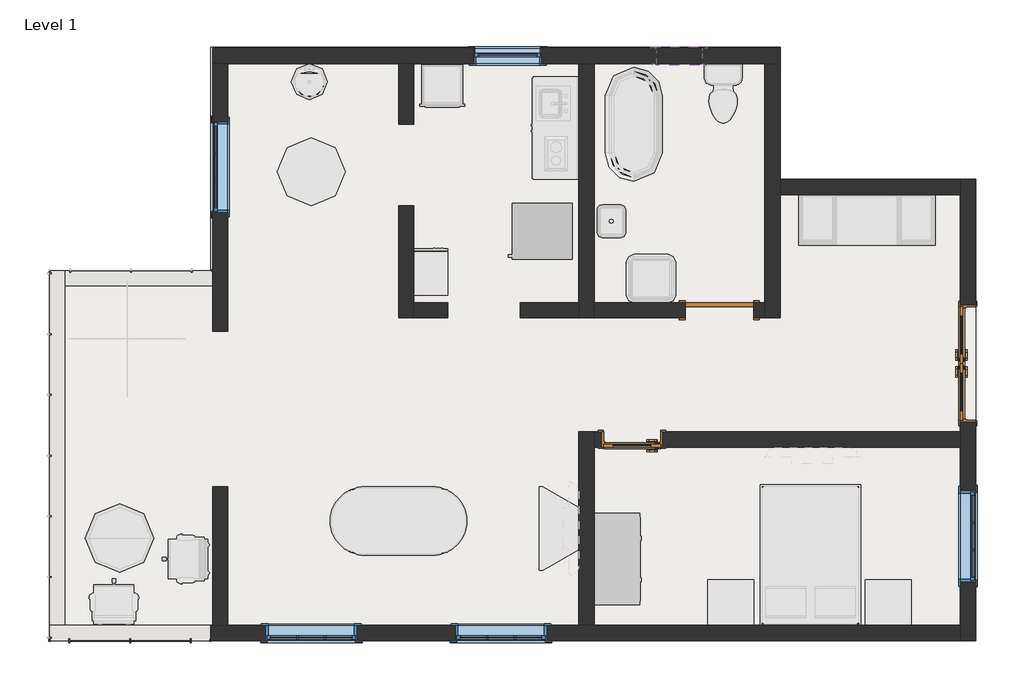
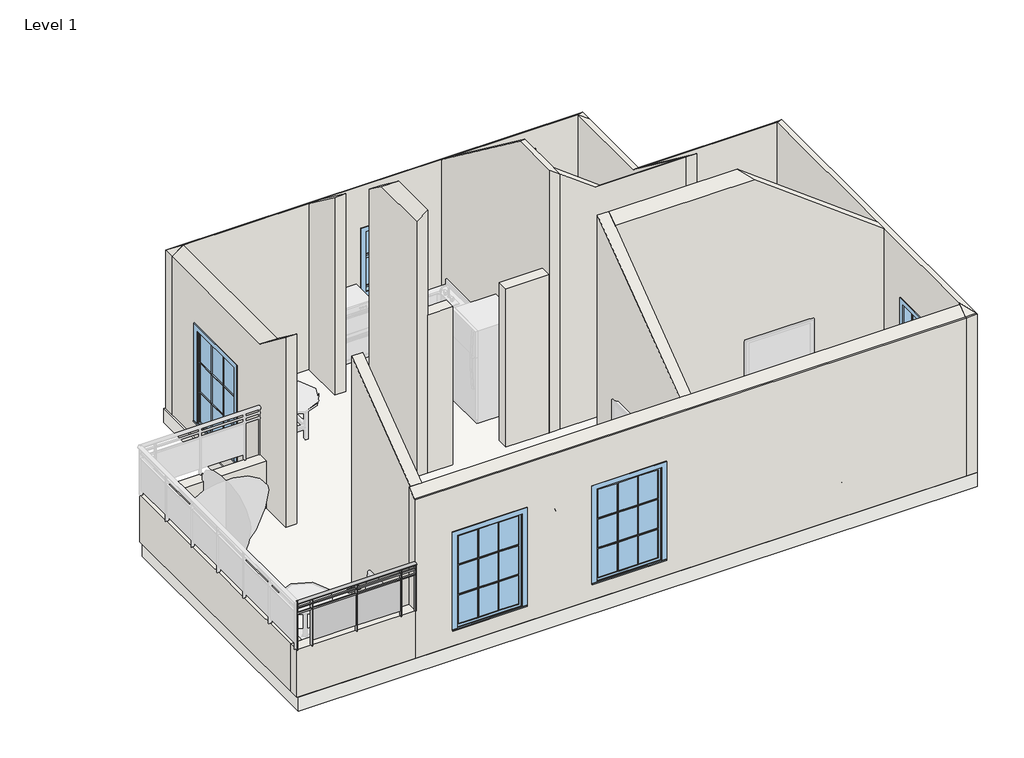
# One storey, part 1 of 2: 18 walls, 6 windows, 3 doors, 1 railing, 1 slab.
"""IFC4 building model written with IfcOpenShell, lengths in millimetres."""

from ifc_helpers import new_model, si_unit, point, frame, origin, origin_with_axes, place, context, project, spatial, polyline, ellipse_curve, trimmed, outline, extrude, faceted_brep, transform, mapped, element, save
from ifc_brep_helpers import plane_surface, extruded_surface, advanced_brep
from components import door_7e6851c9, door_b03bd389, door_54dd4da4, window_5a4e61ec, window_31198920, window_e41d21a6

model = new_model("IFC4")

# Units and contexts
model_context = context("Model", 3, world=origin())
ifc_project = project(units=[si_unit("LENGTHUNIT", "METRE", prefix="MILLI")], contexts=[model_context])

# Site, building, storey
site = spatial("IfcSite", under=ifc_project)
building = spatial("IfcBuilding", under=site)
storey = spatial("IfcBuildingStorey", under=building, Name="Level 1", Elevation=0.0)

# Doors
placement = place(None, origin())
door_shape = door_7e6851c9(model_context)
element("IfcDoor", 1, ObjectType="30\" x 80\"", at=placement, inside=storey, context=model_context, shape_type="MappedRepresentation", body=[
    mapped(door_shape, transform((-12235.0118725, 8691.4702409, 0.0), x_axis=(1.0, 0.0, 0.0), y_axis=(0.0, 1.0, 0.0), z_axis=(0.0, 0.0, 1.0))),
])
door_2_shape = door_b03bd389(model_context)
element("IfcDoor", 2, ObjectType="Door-Exterior-Double-Full Glass-Wood_Clad : 60\" x 80\"", at=placement, inside=storey, context=model_context, shape_type="MappedRepresentation", body=[
    mapped(door_2_shape, transform((-7742.3868725, 9710.6452409, 0.0), x_axis=(0.0, 1.0, 0.0), y_axis=(-1.0, 0.0, 0.0), z_axis=(0.0, 0.0, 1.0))),
])
door_3_shape = door_54dd4da4(model_context)
element("IfcDoor", 3, ObjectType="Single-Flush : 36\" x 84\"", at=placement, inside=storey, context=model_context, shape_type="MappedRepresentation", body=[
    mapped(door_3_shape, transform((-11066.6118725, 10421.8452409, 0.0), x_axis=(1.0, 0.0, 0.0), y_axis=(0.0, 1.0, 0.0), z_axis=(0.0, 0.0, 1.0))),
])

# Railing
element("IfcRailing", 4, ObjectType="Glass Panel - Bottom Fill", at=placement, inside=storey, context=model_context, shape_type="SolidModel", body=[
    advanced_brep(
    [(-17873.8118725, 5964.1452409, 1828.8), (-17873.8118725, 6040.3452409, 1828.8), (-20032.8118725, 5964.1452409, 1828.8), (-20032.8118725, 6040.3452409, 1828.8)],
    [
        (0, 1, ellipse_curve(frame((-17873.8118725, 6002.2452409, 1828.8), z_axis=(1.0, 0.0, 0.0), x_axis=(0.0, 1.0, 0.0)), 38.1, 28.575)),
        (1, 0, ellipse_curve(frame((-17873.8118725, 6002.2452409, 1828.8), z_axis=(1.0, 0.0, 0.0), x_axis=(0.0, 1.0, 0.0)), 38.1, 28.575)),
        (2, 3, ellipse_curve(frame((-20032.8118725, 6002.2452409, 1828.8), z_axis=(-1.0, 0.0, 0.0), x_axis=(0.0, 1.0, 0.0)), 38.1, 28.575)),
        (3, 2, ellipse_curve(frame((-20032.8118725, 6002.2452409, 1828.8), z_axis=(-1.0, 0.0, 0.0), x_axis=(0.0, 1.0, 0.0)), 38.1, 28.575)),
        (0, 2),
        (3, 1),
    ],
    [
        plane_surface(frame((-17873.8118725, 6002.2452409, 1828.8), z_axis=(1.0, 0.0, 0.0), x_axis=(0.0, -1.0, 0.0))),
        plane_surface(frame((-20032.8118725, 6002.2452409, 1828.8), z_axis=(-1.0, 0.0, 0.0), x_axis=(0.0, -1.0, 0.0))),
        extruded_surface(trimmed(ellipse_curve(frame((-20032.8118725, 6002.2452409, 1828.8), z_axis=(1.0, 0.0, 0.0), x_axis=(0.0, 1.0, 0.0)), 38.1, 28.575), [point((-20032.8118725, 5964.1452409, 1828.8))], [point((-20032.8118725, 6040.3452409, 1828.8))], True, "CARTESIAN"), (2159.0, 0.0, 0.0), 2159.0),
        extruded_surface(trimmed(ellipse_curve(frame((-20032.8118725, 6002.2452409, 1828.8), z_axis=(1.0, 0.0, 0.0), x_axis=(0.0, 1.0, 0.0)), 38.1, 28.575), [point((-20032.8118725, 6040.3452409, 1828.8))], [point((-20032.8118725, 5964.1452409, 1828.8))], True, "CARTESIAN"), (2159.0, 0.0, 0.0), 2159.0),
    ],
    [
        (0, [[1, 2]]),
        (1, [[3, 4]]),
        (2, [[-1, 5, -4, 6]]),
        (3, [[-2, -6, -3, -5]]),
    ],
),
    extrude(outline(polyline([(-17873.8118725, 6014.9452409), (-17873.8118725, 5989.5452409), (-20032.8118725, 5989.5452409), (-20032.8118725, 6014.9452409), (-17873.8118725, 6014.9452409)])), frame((0.0, 0.0, 1714.5), z_axis=(0.0, 0.0, 1.0), x_axis=(1.0, 0.0, 0.0)), (0.0, 0.0, 1.0), 25.4),
    extrude(outline(polyline([(-17873.8118725, 6014.9452409), (-17873.8118725, 5989.5452409), (-20032.8118725, 5989.5452409), (-20032.8118725, 6014.9452409), (-17873.8118725, 6014.9452409)])), frame((0.0, 0.0, 1612.9), z_axis=(0.0, 0.0, 1.0), x_axis=(1.0, 0.0, 0.0)), (0.0, 0.0, 1.0), 25.4),
    extrude(outline(polyline([(-19759.7618725, 6027.6452409), (-19759.7618725, 5976.8452409), (-19772.4618725, 5976.8452409), (-19772.4618725, 6027.6452409), (-19759.7618725, 6027.6452409)])), frame((0.0, 0.0, 914.4), z_axis=(0.0, 0.0, 1.0), x_axis=(1.0, 0.0, 0.0)), (0.0, 0.0, 1.0), 885.6788223),
    extrude(outline(polyline([(-18953.3118725, 5995.7100839), (-19766.1118725, 5995.7100839), (-19766.1118725, 6002.0600839), (-18953.3118725, 6002.0600839), (-18953.3118725, 5995.7100839)])), frame((0.0, 0.0, 1016.0), z_axis=(0.0, 0.0, 1.0), x_axis=(1.0, 0.0, 0.0)), (0.0, 0.0, 1.0), 596.9),
    extrude(outline(polyline([(-18946.9618725, 6027.6452409), (-18946.9618725, 5976.8452409), (-18959.6618725, 5976.8452409), (-18959.6618725, 6027.6452409), (-18946.9618725, 6027.6452409)])), frame((0.0, 0.0, 914.4), z_axis=(0.0, 0.0, 1.0), x_axis=(1.0, 0.0, 0.0)), (0.0, 0.0, 1.0), 885.6788223),
    extrude(outline(polyline([(-18140.5118725, 5995.7100839), (-18953.3118725, 5995.7100839), (-18953.3118725, 6002.0600839), (-18140.5118725, 6002.0600839), (-18140.5118725, 5995.7100839)])), frame((0.0, 0.0, 1016.0), z_axis=(0.0, 0.0, 1.0), x_axis=(1.0, 0.0, 0.0)), (0.0, 0.0, 1.0), 596.9),
    extrude(outline(polyline([(-18134.1618725, 6027.6452409), (-18134.1618725, 5976.8452409), (-18146.8618725, 5976.8452409), (-18146.8618725, 6027.6452409), (-18134.1618725, 6027.6452409)])), frame((0.0, 0.0, 914.4), z_axis=(0.0, 0.0, 1.0), x_axis=(1.0, 0.0, 0.0)), (0.0, 0.0, 1.0), 885.6788223),
    extrude(outline(polyline([(-20020.1118725, 6011.7702409), (-20020.1118725, 5992.7202409), (-20039.1618725, 5992.7202409), (-20039.1618725, 6011.7702409), (-20020.1118725, 6011.7702409)])), frame((0.0, 0.0, 914.4), z_axis=(0.0, 0.0, 1.0), x_axis=(1.0, 0.0, 0.0)), (0.0, 0.0, 1.0), 885.6788223),
    extrude(outline(polyline([(-17867.4618725, 6011.7702409), (-17867.4618725, 5992.7202409), (-17886.5118725, 5992.7202409), (-17886.5118725, 6011.7702409), (-17867.4618725, 6011.7702409)])), frame((0.0, 0.0, 914.4), z_axis=(0.0, 0.0, 1.0), x_axis=(1.0, 0.0, 0.0)), (0.0, 0.0, 1.0), 885.6788223),
])

# Slab
element("IfcSlab", 5, ObjectType="Wood Joist 10\" - Ceramic Tile", at=placement, inside=storey, context=model_context, shape_type="SweptSolid", body=[
    extrude(outline(polyline([(-20007.4118725, 10923.4952409), (-17873.8118725, 10923.4952409), (-17873.8118725, 13946.0952409), (-10253.8118725, 13946.0952409), (-10253.8118725, 12174.4452409), (-7637.6118725, 12174.4452409), (-7637.6118725, 10542.4952409), (-7637.6118725, 6002.2452409), (-20007.4118725, 6002.2452409), (-20007.4118725, 10923.4952409)])), frame((0.0, 0.0, -273.05), z_axis=(0.0, 0.0, 1.0), x_axis=(1.0, 0.0, 0.0)), (0.0, 0.0, 1.0), 273.05),
])

# Walls
element("IfcWall", 6, ObjectType="Generic - 8\"", at=placement, inside=storey, context=model_context, shape_type="Brep", body=[
    faceted_brep([(-7840.8118725, 6205.4452409, 0.0), (-12743.0118725, 6205.4452409, 0.0), (-12946.2118725, 6205.4452409, 0.0), (-17645.2118725, 6205.4452409, 0.0), (-17848.4118725, 6205.4452409, 0.0), (-17873.8118725, 6205.4452409, 0.0), (-17873.8118725, 6205.4452409, 914.4), (-17873.8118725, 6205.4452409, 3176.5875), (-17848.4118725, 6205.4452409, 3176.5875), (-17645.2118725, 6205.4452409, 3176.5875), (-12946.2118725, 6205.4452409, 3176.5875), (-12743.0118725, 6205.4452409, 3176.5875), (-7840.8118725, 6205.4452409, 3176.5875), (-17137.2118725, 6205.4452409, 2133.6), (-17137.2118725, 6205.4452409, 304.8), (-15918.0118725, 6205.4452409, 304.8), (-15918.0118725, 6205.4452409, 2133.6), (-14597.2118725, 6205.4452409, 2133.6), (-14597.2118725, 6205.4452409, 304.8), (-13378.0118725, 6205.4452409, 304.8), (-13378.0118725, 6205.4452409, 2133.6), (-7840.8118725, 6002.2452409, 0.0), (-7840.8118725, 6002.2452409, 3048.0), (-17873.8118725, 6002.2452409, 3048.0), (-17873.8118725, 6002.2452409, 914.4), (-17873.8118725, 6002.2452409, 0.0), (-17137.2118725, 6002.2452409, 2133.6), (-15918.0118725, 6002.2452409, 2133.6), (-15918.0118725, 6002.2452409, 304.8), (-17137.2118725, 6002.2452409, 304.8), (-14597.2118725, 6002.2452409, 2133.6), (-13378.0118725, 6002.2452409, 2133.6), (-13378.0118725, 6002.2452409, 304.8), (-14597.2118725, 6002.2452409, 304.8), (-17873.8118725, 6033.9952409, 3048.0), (-7840.8118725, 6033.9952409, 3048.0)], [[[0, 1, 2, 3, 4, 5, 6, 7, 8, 9, 10, 11, 12], [13, 14, 15, 16], [17, 18, 19, 20]], [[21, 22, 23, 24, 25], [26, 27, 28, 29], [30, 31, 32, 33]], [[5, 4, 3, 2, 1, 0, 21, 25]], [[7, 6, 5, 25, 24, 23, 34]], [[0, 12, 35, 22, 21]], [[34, 23, 22, 35]], [[12, 11, 10, 9, 8, 7, 34, 35]], [[14, 13, 26, 29]], [[15, 14, 29, 28]], [[16, 15, 28, 27]], [[13, 16, 27, 26]], [[18, 17, 30, 33]], [[19, 18, 33, 32]], [[20, 19, 32, 31]], [[17, 20, 31, 30]]]),
])
element("IfcWall", 7, ObjectType="Generic - 8\"", at=placement, inside=storey, context=model_context, shape_type="Brep", body=[
    faceted_brep([(-19829.6118725, 6205.4452409, 0.0), (-19829.6118725, 10752.0452409, 0.0), (-19829.6118725, 10955.2452409, 0.0), (-19829.6118725, 10955.2452409, 914.4), (-19829.6118725, 10752.0452409, 914.4), (-19829.6118725, 6205.4452409, 914.4), (-20032.8118725, 6205.4452409, 0.0), (-20032.8118725, 6205.4452409, 914.4), (-20032.8118725, 10955.2452409, 914.4), (-20032.8118725, 10955.2452409, 0.0)], [[[0, 1, 2, 3, 4, 5]], [[6, 7, 8, 9]], [[2, 1, 0, 6, 9]], [[5, 4, 3, 8, 7]], [[0, 5, 7, 6]], [[3, 2, 9, 8]]]),
])
element("IfcWall", 8, ObjectType="Generic - 8\"", at=placement, inside=storey, context=model_context, shape_type="SweptSolid", body=[
    extrude(outline(polyline([(12174.4452409, 3048.0), (12174.4452409, 0.0), (11971.2452409, 0.0), (11971.2452409, 3200.4), (12174.4452409, 3048.0)])), frame((-10253.8118725, 0.0, 0.0), z_axis=(1.0, 0.0, 0.0), x_axis=(0.0, 1.0, 0.0)), (0.0, 0.0, 1.0), 2413.0),
])
element("IfcWall", 9, ObjectType="Generic - 8\"", at=placement, inside=storey, context=model_context, shape_type="Brep", body=[
    faceted_brep([(-10253.8118725, 10320.2452409, 0.0), (-10253.8118725, 11971.2452409, 0.0), (-10253.8118725, 12174.4452409, 0.0), (-10253.8118725, 13723.8452409, 0.0), (-10253.8118725, 13723.8452409, 3048.0), (-10253.8118725, 12174.4452409, 3048.0), (-10253.8118725, 11971.2452409, 3200.4), (-10253.8118725, 10320.2452409, 4438.65), (-10457.0118725, 10320.2452409, 0.0), (-10457.0118725, 10320.2452409, 4438.65), (-10457.0118725, 10523.4452409, 4286.25), (-10457.0118725, 11971.2452409, 3200.4), (-10457.0118725, 13723.8452409, 3200.4), (-10457.0118725, 13723.8452409, 0.0), (-10457.0118725, 10523.4452409, 0.0)], [[[0, 1, 2, 3, 4, 5, 6, 7]], [[8, 9, 10, 11, 12, 13, 14]], [[3, 2, 1, 0, 8, 14, 13]], [[4, 3, 13, 12]], [[0, 7, 9, 8]], [[7, 6, 5, 11, 10, 9]], [[5, 4, 12, 11]]]),
])
element("IfcWall", 10, ObjectType="Generic - 8\"", at=placement, inside=storey, context=model_context, shape_type="Brep", body=[
    faceted_brep([(-12946.2118725, 13723.8452409, 0.0), (-12946.2118725, 10523.4452409, 0.0), (-12946.2118725, 10320.2452409, 0.0), (-12946.2118725, 10320.2452409, 3048.0), (-12946.2118725, 10320.2452409, 5067.3), (-12946.2118725, 11234.6452409, 5067.3), (-12946.2118725, 13723.8452409, 3200.4), (-12743.0118725, 13723.8452409, 0.0), (-12743.0118725, 13723.8452409, 3200.4), (-12743.0118725, 11437.8452409, 4914.9), (-12743.0118725, 10523.4452409, 4914.9), (-12743.0118725, 10320.2452409, 4914.9), (-12743.0118725, 10320.2452409, 0.0), (-12743.0118725, 10523.4452409, 0.0)], [[[0, 1, 2, 3, 4, 5, 6]], [[7, 8, 9, 10, 11, 12, 13]], [[2, 1, 0, 7, 13, 12]], [[0, 6, 8, 7]], [[6, 5, 9, 8]], [[5, 4, 11, 10, 9]], [[4, 3, 2, 12, 11]]]),
])
element("IfcWall", 11, ObjectType="Generic - 8\"", at=placement, inside=storey, context=model_context, shape_type="Brep", body=[
    faceted_brep([(-17848.4118725, 13723.8452409, 0.0), (-17848.4118725, 10955.2452409, 0.0), (-17848.4118725, 10752.0452409, 0.0), (-17848.4118725, 10142.4452409, 0.0), (-17848.4118725, 10142.4452409, 3657.6), (-17848.4118725, 10955.2452409, 3048.0), (-17848.4118725, 13723.8452409, 3048.0), (-17848.4118725, 12949.1452409, 2133.6), (-17848.4118725, 11729.9452409, 2133.6), (-17848.4118725, 11729.9452409, 304.8), (-17848.4118725, 12949.1452409, 304.8), (-17645.2118725, 13723.8452409, 0.0), (-17645.2118725, 13723.8452409, 3200.4), (-17645.2118725, 10752.0452409, 3200.4), (-17645.2118725, 10142.4452409, 3657.6), (-17645.2118725, 10142.4452409, 0.0), (-17645.2118725, 12949.1452409, 2133.6), (-17645.2118725, 12949.1452409, 304.8), (-17645.2118725, 11729.9452409, 304.8), (-17645.2118725, 11729.9452409, 2133.6)], [[[0, 1, 2, 3, 4, 5, 6], [7, 8, 9, 10]], [[11, 12, 13, 14, 15], [16, 17, 18, 19]], [[3, 2, 1, 0, 11, 15]], [[4, 3, 15, 14]], [[0, 6, 12, 11]], [[6, 5, 13, 12]], [[5, 4, 14, 13]], [[17, 16, 7, 10]], [[18, 17, 10, 9]], [[19, 18, 9, 8]], [[16, 19, 8, 7]]]),
])
element("IfcWall", 12, ObjectType="Generic - 8\"", at=placement, inside=storey, context=model_context, shape_type="SweptSolid", body=[
    extrude(outline(polyline([(-19829.6118725, 10955.2452409), (-17848.4118725, 10955.2452409), (-17848.4118725, 10752.0452409), (-19829.6118725, 10752.0452409), (-19829.6118725, 10955.2452409)])), origin_with_axes(), (0.0, 0.0, 1.0), 914.4),
])
element("IfcWall", 13, ObjectType="Generic - 8\"", at=placement, inside=storey, context=model_context, shape_type="Brep", body=[
    faceted_brep([(-17848.4118725, 13723.8452409, 0.0), (-17645.2118725, 13723.8452409, 0.0), (-15359.2118725, 13723.8452409, 0.0), (-15156.0118725, 13723.8452409, 0.0), (-12946.2118725, 13723.8452409, 0.0), (-12743.0118725, 13723.8452409, 0.0), (-10457.0118725, 13723.8452409, 0.0), (-10253.8118725, 13723.8452409, 0.0), (-10253.8118725, 13723.8452409, 3048.0), (-10457.0118725, 13723.8452409, 3200.4), (-12743.0118725, 13723.8452409, 3200.4), (-12946.2118725, 13723.8452409, 3200.4), (-15156.0118725, 13723.8452409, 3200.4), (-15359.2118725, 13723.8452409, 3200.4), (-17645.2118725, 13723.8452409, 3200.4), (-17848.4118725, 13723.8452409, 3048.0), (-13441.5118725, 13723.8452409, 2336.8), (-13441.5118725, 13723.8452409, 1117.6), (-14355.9118725, 13723.8452409, 1117.6), (-14355.9118725, 13723.8452409, 2336.8), (-11295.2118725, 13723.8452409, 2768.6), (-11295.2118725, 13723.8452409, 2159.0), (-11904.8118725, 13723.8452409, 2159.0), (-11904.8118725, 13723.8452409, 2768.6), (-17848.4118725, 13927.0452409, 0.0), (-17848.4118725, 13927.0452409, 3048.0), (-10253.8118725, 13927.0452409, 3048.0), (-10253.8118725, 13927.0452409, 0.0), (-13441.5118725, 13927.0452409, 2336.8), (-14355.9118725, 13927.0452409, 2336.8), (-14355.9118725, 13927.0452409, 1117.6), (-13441.5118725, 13927.0452409, 1117.6), (-11295.2118725, 13927.0452409, 2768.6), (-11904.8118725, 13927.0452409, 2768.6), (-11904.8118725, 13927.0452409, 2159.0), (-11295.2118725, 13927.0452409, 2159.0)], [[[0, 1, 2, 3, 4, 5, 6, 7, 8, 9, 10, 11, 12, 13, 14, 15], [16, 17, 18, 19], [20, 21, 22, 23]], [[24, 25, 26, 27], [28, 29, 30, 31], [32, 33, 34, 35]], [[7, 6, 5, 4, 3, 2, 1, 0, 24, 27]], [[0, 15, 25, 24]], [[8, 7, 27, 26]], [[15, 14, 25]], [[14, 13, 12, 11, 10, 9, 26, 25]], [[9, 8, 26]], [[17, 16, 28, 31]], [[18, 17, 31, 30]], [[19, 18, 30, 29]], [[16, 19, 29, 28]], [[21, 20, 32, 35]], [[22, 21, 35, 34]], [[23, 22, 34, 33]], [[20, 23, 33, 32]]]),
])
element("IfcWall", 14, ObjectType="Generic - 8\"", at=placement, inside=storey, context=model_context, shape_type="Brep", body=[
    faceted_brep([(-7840.8118725, 6002.2452409, 0.0), (-7840.8118725, 6002.2452409, 3048.0), (-7840.8118725, 6033.9952409, 3048.0), (-7840.8118725, 6205.4452409, 3176.5875), (-7840.8118725, 6237.1952409, 3200.4), (-7840.8118725, 8593.0452409, 3200.4), (-7840.8118725, 8796.2452409, 3200.4), (-7840.8118725, 11971.2452409, 3200.4), (-7840.8118725, 12174.4452409, 3048.0), (-7840.8118725, 12174.4452409, 0.0), (-7840.8118725, 11971.2452409, 0.0), (-7840.8118725, 10498.0452409, 0.0), (-7840.8118725, 10498.0452409, 2057.4), (-7840.8118725, 8923.2452409, 2057.4), (-7840.8118725, 8923.2452409, 0.0), (-7840.8118725, 8796.2452409, 0.0), (-7840.8118725, 8593.0452409, 0.0), (-7840.8118725, 6205.4452409, 0.0), (-7840.8118725, 6789.6452409, 2133.6), (-7840.8118725, 6789.6452409, 304.8), (-7840.8118725, 8008.8452409, 304.8), (-7840.8118725, 8008.8452409, 2133.6), (-7637.6118725, 6002.2452409, 3048.0), (-7637.6118725, 6002.2452409, 0.0), (-7637.6118725, 8923.2452409, 0.0), (-7637.6118725, 8923.2452409, 2057.4), (-7637.6118725, 10498.0452409, 2057.4), (-7637.6118725, 10498.0452409, 0.0), (-7637.6118725, 12174.4452409, 0.0), (-7637.6118725, 12174.4452409, 3048.0), (-7637.6118725, 6033.9952409, 3048.0), (-7637.6118725, 6789.6452409, 2133.6), (-7637.6118725, 8008.8452409, 2133.6), (-7637.6118725, 8008.8452409, 304.8), (-7637.6118725, 6789.6452409, 304.8)], [[[0, 1, 2, 3, 4, 5, 6, 7, 8, 9, 10, 11, 12, 13, 14, 15, 16, 17], [18, 19, 20, 21]], [[22, 23, 24, 25, 26, 27, 28, 29, 30], [31, 32, 33, 34]], [[23, 0, 17, 16, 15, 14, 24]], [[9, 28, 27, 11, 10]], [[1, 0, 23, 22]], [[9, 8, 29, 28]], [[26, 12, 11, 27]], [[12, 26, 25, 13]], [[13, 25, 24, 14]], [[1, 22, 30, 2]], [[29, 8, 7]], [[30, 29, 7, 6, 5, 4]], [[4, 3, 2, 30]], [[19, 18, 31, 34]], [[20, 19, 34, 33]], [[21, 20, 33, 32]], [[18, 21, 32, 31]]]),
])
element("IfcWall", 15, ObjectType="Generic - 8\"", at=placement, inside=storey, context=model_context, shape_type="Brep", body=[
    faceted_brep([(-12743.0118725, 8593.0452409, 4967.2875), (-12743.0118725, 8593.0452409, 0.0), (-12641.4118725, 8593.0452409, 0.0), (-12641.4118725, 8593.0452409, 2057.4), (-11828.6118725, 8593.0452409, 2057.4), (-11828.6118725, 8593.0452409, 0.0), (-7840.8118725, 8593.0452409, 0.0), (-7840.8118725, 8593.0452409, 3200.4), (-10196.6618725, 8593.0452409, 4967.2875), (-12743.0118725, 8796.2452409, 0.0), (-12743.0118725, 8796.2452409, 5119.6875), (-10399.8618725, 8796.2452409, 5119.6875), (-7840.8118725, 8796.2452409, 3200.4), (-7840.8118725, 8796.2452409, 0.0), (-11828.6118725, 8796.2452409, 0.0), (-11828.6118725, 8796.2452409, 2057.4), (-12641.4118725, 8796.2452409, 2057.4), (-12641.4118725, 8796.2452409, 0.0)], [[[0, 1, 2, 3, 4, 5, 6, 7, 8]], [[9, 10, 11, 12, 13, 14, 15, 16, 17]], [[1, 9, 17, 2]], [[13, 6, 5, 14]], [[1, 0, 10, 9]], [[7, 6, 13, 12]], [[4, 15, 14, 5]], [[15, 4, 3, 16]], [[16, 3, 2, 17]], [[10, 0, 8, 11]], [[7, 12, 11, 8]]]),
])
element("IfcWall", 16, ObjectType="Generic - 8\"", at=placement, inside=storey, context=model_context, shape_type="Brep", body=[
    faceted_brep([(-10609.4118725, 10320.2452409, 2133.6), (-10609.4118725, 10320.2452409, 0.0), (-10457.0118725, 10320.2452409, 0.0), (-10457.0118725, 10320.2452409, 4438.65), (-12108.0118725, 10320.2452409, 4438.65), (-12743.0118725, 10320.2452409, 4914.9), (-12743.0118725, 10320.2452409, 0.0), (-11523.8118725, 10320.2452409, 0.0), (-11523.8118725, 10320.2452409, 2133.6), (-10457.0118725, 10523.4452409, 0.0), (-10609.4118725, 10523.4452409, 0.0), (-10609.4118725, 10523.4452409, 2133.6), (-11523.8118725, 10523.4452409, 2133.6), (-11523.8118725, 10523.4452409, 0.0), (-12743.0118725, 10523.4452409, 0.0), (-12743.0118725, 10523.4452409, 4914.9), (-11904.8118725, 10523.4452409, 4286.25), (-10457.0118725, 10523.4452409, 4286.25)], [[[0, 1, 2, 3, 4, 5, 6, 7, 8]], [[9, 10, 11, 12, 13, 14, 15, 16, 17]], [[7, 6, 14, 13]], [[2, 1, 10, 9]], [[3, 2, 9, 17]], [[6, 5, 15, 14]], [[11, 10, 1, 0]], [[12, 11, 0, 8]], [[13, 12, 8, 7]], [[5, 4, 16, 15]], [[4, 3, 17, 16]]]),
])
element("IfcWall", 17, ObjectType="Generic - 8\"", at=placement, inside=storey, context=model_context, shape_type="SweptSolid", body=[
    extrude(outline(polyline([(13723.8452409, 0.0), (12911.0452409, 0.0), (12911.0452409, 3810.0), (13723.8452409, 3200.4), (13723.8452409, 0.0)])), frame((-15359.2118725, 0.0, 0.0), z_axis=(1.0, 0.0, 0.0), x_axis=(0.0, 1.0, 0.0)), (0.0, 0.0, 1.0), 203.2),
])
element("IfcWall", 18, ObjectType="Generic - 8\"", at=placement, inside=storey, context=model_context, shape_type="Brep", body=[
    faceted_brep([(-15359.2118725, 11818.8452409, 0.0), (-15359.2118725, 10320.2452409, 0.0), (-15359.2118725, 10320.2452409, 4914.9), (-15359.2118725, 11437.8452409, 4914.9), (-15359.2118725, 11818.8452409, 4629.15), (-15156.0118725, 11818.8452409, 0.0), (-15156.0118725, 11818.8452409, 4629.15), (-15156.0118725, 11234.6452409, 5067.3), (-15156.0118725, 10320.2452409, 5067.3), (-15156.0118725, 10320.2452409, 3048.0), (-15156.0118725, 10320.2452409, 0.0), (-15156.0118725, 10523.4452409, 0.0)], [[[0, 1, 2, 3, 4]], [[5, 6, 7, 8, 9, 10, 11]], [[1, 0, 5, 11, 10]], [[0, 4, 6, 5]], [[2, 1, 10, 9, 8]], [[4, 3, 7, 6]], [[3, 2, 8, 7]]]),
])
element("IfcWall", 19, ObjectType="Generic - 8\"", at=placement, inside=storey, context=model_context, shape_type="Brep", body=[
    faceted_brep([(-17873.8118725, 6205.4452409, 0.0), (-19829.6118725, 6205.4452409, 0.0), (-20032.8118725, 6205.4452409, 0.0), (-20032.8118725, 6205.4452409, 914.4), (-19829.6118725, 6205.4452409, 914.4), (-17873.8118725, 6205.4452409, 914.4), (-17873.8118725, 6002.2452409, 0.0), (-17873.8118725, 6002.2452409, 914.4), (-20032.8118725, 6002.2452409, 914.4), (-20032.8118725, 6002.2452409, 0.0)], [[[0, 1, 2, 3, 4, 5]], [[6, 7, 8, 9]], [[2, 1, 0, 6, 9]], [[5, 4, 3, 8, 7]], [[0, 5, 7, 6]], [[3, 2, 9, 8]]]),
])
element("IfcWall", 20, ObjectType="Generic - 8\"", at=placement, inside=storey, context=model_context, shape_type="SweptSolid", body=[
    extrude(outline(polyline([(8059.6452409, 0.0), (6205.4452409, 0.0), (6205.4452409, 3176.5875), (8059.6452409, 4567.2375), (8059.6452409, 0.0)])), frame((-17848.4118725, 0.0, 0.0), z_axis=(1.0, 0.0, 0.0), x_axis=(0.0, 1.0, 0.0)), (0.0, 0.0, 1.0), 203.2),
])
element("IfcWall", 21, ObjectType="Generic - 8\"", at=placement, inside=storey, context=model_context, shape_type="Brep", body=[
    faceted_brep([(-12946.2118725, 8796.2452409, 0.0), (-12946.2118725, 6205.4452409, 0.0), (-12946.2118725, 6205.4452409, 3176.5875), (-12946.2118725, 8796.2452409, 5119.6875), (-12743.0118725, 8796.2452409, 0.0), (-12743.0118725, 8796.2452409, 5119.6875), (-12743.0118725, 8593.0452409, 4967.2875), (-12743.0118725, 6205.4452409, 3176.5875), (-12743.0118725, 6205.4452409, 0.0), (-12743.0118725, 8593.0452409, 0.0)], [[[0, 1, 2, 3]], [[4, 5, 6, 7, 8, 9]], [[1, 0, 4, 9, 8]], [[0, 3, 5, 4]], [[2, 1, 8, 7]], [[3, 2, 7, 6, 5]]]),
])
element("IfcWall", 22, ObjectType="Generic - 8\"", at=placement, inside=storey, context=model_context, shape_type="SweptSolid", body=[
    extrude(outline(polyline([(-13733.6118725, 10523.4452409), (-12946.2118725, 10523.4452409), (-12946.2118725, 10320.2452409), (-13733.6118725, 10320.2452409), (-13733.6118725, 10523.4452409)])), origin_with_axes(), (0.0, 0.0, 1.0), 3048.0),
])
element("IfcWall", 23, ObjectType="Generic - 8\"", at=placement, inside=storey, context=model_context, shape_type="SweptSolid", body=[
    extrude(outline(polyline([(-15156.0118725, 10523.4452409), (-14698.8118725, 10523.4452409), (-14698.8118725, 10320.2452409), (-15156.0118725, 10320.2452409), (-15156.0118725, 10523.4452409)])), origin_with_axes(), (0.0, 0.0, 1.0), 3048.0),
])

# Windows
window_shape = window_5a4e61ec(model_context)
element("IfcWindow", 24, ObjectType="Casement 3x3 with Trim : 48\" x 72\"", at=placement, inside=storey, context=model_context, shape_type="MappedRepresentation", body=[
    mapped(window_shape, transform((-16527.6118725, 6103.8452409, 0.0), x_axis=(-1.0, 0.0, 0.0), y_axis=(0.0, -1.0, 0.0), z_axis=(0.0, 0.0, 1.0))),
])
element("IfcWindow", 25, ObjectType="Casement 3x3 with Trim : 48\" x 72\"", at=placement, inside=storey, context=model_context, shape_type="MappedRepresentation", body=[
    mapped(window_shape, transform((-13987.6118725, 6103.8452409, 0.0), x_axis=(-1.0, 0.0, 0.0), y_axis=(0.0, -1.0, 0.0), z_axis=(0.0, 0.0, 1.0))),
])
element("IfcWindow", 26, ObjectType="Casement 3x3 with Trim : 48\" x 72\"", at=placement, inside=storey, context=model_context, shape_type="MappedRepresentation", body=[
    mapped(window_shape, transform((-7739.2118725, 7399.2452409, 0.0), x_axis=(0.0, -1.0, 0.0), y_axis=(1.0, 0.0, 0.0), z_axis=(0.0, 0.0, 1.0))),
])
element("IfcWindow", 27, ObjectType="Casement 3x3 with Trim : 48\" x 72\"", at=placement, inside=storey, context=model_context, shape_type="MappedRepresentation", body=[
    mapped(window_shape, transform((-17746.8118725, 12339.5452409, 0.0), x_axis=(0.0, 1.0, 0.0), y_axis=(-1.0, 0.0, 0.0), z_axis=(0.0, 0.0, 1.0))),
])
window_2_shape = window_31198920(model_context)
element("IfcWindow", 28, ObjectType="Double Hung with Trim : 36\" x 48\"", at=placement, inside=storey, context=model_context, shape_type="MappedRepresentation", body=[
    mapped(window_2_shape, transform((-13898.7118725, 13825.4452409, 203.2), x_axis=(1.0, 0.0, 0.0), y_axis=(0.0, 1.0, 0.0), z_axis=(0.0, 0.0, 1.0))),
])
window_3_shape = window_e41d21a6(model_context)
element("IfcWindow", 29, ObjectType="Transom with Trim : 24\" x 24\"", at=placement, inside=storey, context=model_context, shape_type="MappedRepresentation", body=[
    mapped(window_3_shape, transform((-11561.9118725, 13825.4452409, 0.0), x_axis=(1.0, 0.0, 0.0), y_axis=(0.0, 1.0, 0.0), z_axis=(0.0, 0.0, 1.0))),
])

save(model, "model.ifc")

# Revit data of these elements
# Type "30\" x 80\""
#   Type Mark = "9"
#   Assembly Code = "B2030100"
#   Analytic Construction = "French door, wood frame with single glass"
#   Top Rail = 0' - 4 3/4"
#   Threshold Offset [instance default] = 0' - 0 1/2"
#   Thickness = 0' - 1 3/8"
#   Thermal Resistance (R) = 1.0696 (h·ft²·°F)/BTU
#   Swing Angle [instance default] = 90.00°
#   Stiles = 0' - 4 3/4"
#   Rough Width = 2' - 8"
#   Rough Height = 6' - 9"
#   Lock Rail = 0' - 7 1/8"
#   Height = 6' - 8"
#   Width = 2' - 6"
#   Heat Transfer Coefficient (U) = 0.9350 BTU/(h·ft²·°F)
#   Door Offset [instance default] = 0' - 0"
#   Bottom Rail = 0' - 9 1/2"
#   Threshold [instance default] = yes
#   Function = 1
#   Exterior Trim [instance default] = yes
#   Trim Material = Cherry
#   Threshold Material = Cherry
#   Panel Material = Cherry
#   Glazing = Glass
#   Frame Material = Cherry
#   Door Handle Material = Aluminum
#   Visual Light Transmittance = 0
#   Solar Heat Gain Coefficient = 0
#   Wall Closure = (empty or 0)
#   Construction Type = (empty or 0)
# Type "Door-Exterior-Double-Full Glass-Wood_Clad : 60\" x 80\""
#   Type Mark = "8"
#   Assembly Code = "B2030100"
#   Analytic Construction = "French door, wood frame with double glass"
#   Top Rail = 0' - 4 11/16"
#   Threshold Offset [instance default] = 0' - 0 1/2"
#   Thickness = 0' - 1 3/8"
#   Thermal Resistance (R) = 1.9158 (h·ft²·°F)/BTU
#   Swing Angle [instance default] = 90.00°
#   Stiles = 0' - 4 3/4"
#   Rough Width = 5' - 2"
#   Rough Height = 6' - 9"
#   Panel Width = 2' - 6"
#   Door Offset [instance default] = 0' - 0"
#   Height = 6' - 8"
#   Width = 5' - 0"
#   Heat Transfer Coefficient (U) = 0.5220 BTU/(h·ft²·°F)
#   Bottom Rail = 0' - 9 1/8"
#   Exterior Trim [instance default] = yes
#   Threshold [instance default] = yes
#   Show Grill [instance default] = yes
#   Function = 1
#   Trim Material = Cherry
#   Threshold Material = Cherry
#   Panel Material = Cherry
#   Glazing = Glass
#   Frame Material = Cherry
#   Door Handle Material = Aluminum
#   Visual Light Transmittance = 0
#   Solar Heat Gain Coefficient = 0
#   Wall Closure = (empty or 0)
#   Construction Type = (empty or 0)
# Type "Single-Flush : 36\" x 84\""
#   Type Mark = "1"
#   Construction Type Id = "MDOOR"
#   Assembly Code = "C1020"
#   Analytic Construction = "Metal"
#   Thickness = 0' - 2"
#   Heat Transfer Coefficient (U) = 0.651978 BTU/(h·ft²·°F)
#   Height = 7' - 0"
#   Trim Projection Ext = 0' - 1"
#   Trim Projection Int = 0' - 1"
#   Trim Width = 0' - 3"
#   Width = 3' - 0"
#   Define Thermal Properties by = 1
#   Door Material = Door - Panel
#   Frame Material = Door - Frame
#   Visual Light Transmittance = 0
#   Solar Heat Gain Coefficient = 0
#   Function = (empty or 0)
#   Wall Closure = (empty or 0)
# Type "Glass Panel - Bottom Fill"
#   Assembly Code = "C2010400"
#   built-in parameter 1008612 = 0.0416667 (stored number, unit not read)
#   built-in parameter 1008611 = 0.0416667 (stored number, unit not read)
#   built-in parameter 1008609 = 0.333333 (stored number, unit not read)
#   built-in parameter 1008604 = 0.166667 (stored number, unit not read)
#   built-in parameter 1008603 = 0.166667 (stored number, unit not read)
#   Railing Height = 3' - 0"
#   built-in parameter 1008630 = 2
#   built-in parameter 1008610 = 2
#   built-in parameter 1008618 = Baluster - Square : 3/4"
# Type "Wood Joist 10\" - Ceramic Tile"
#   Assembly Code = "B1010"
#   Function = 0
#   Layers, outside or top first: 0' - 0 1/4" "Tile, Mosaic, Gray" (function 5); 0' - 0 1/2" "Concrete, Cast-in-Place gray" (function 4); 0' - 0 3/4" "Plywood, Sheathing" (function 1); 0' - 9 1/4" "Structure, Wood Joist/Rafter Layer" (function 1)
# Type "Generic - 8\""
#   Assembly Code = "B2010"
#   Layers, outside or top first: 0' - 8" "Brick, Common" (function 1)
# Type "Casement 3x3 with Trim : 48\" x 72\""
#   Type Mark = "12"
#   Construction Type Id = "GSP4R"
#   Assembly Code = "B2020100"
#   Analytic Construction = "1/8 in Pilkington single glazing"
#   Visual Light Transmittance = 0.9
#   Solar Heat Gain Coefficient = 0.78
#   Heat Transfer Coefficient (U) = 0.6496 BTU/(h·ft²·°F)
#   Height = 6' - 0"
#   Default Sill Height = 1' - 0"
#   Trim Projection - Ext. = 0' - 0 1/2"
#   Trim Projection - Int. = 0' - 0 3/4"
#   Trim Width - Exterior = 0' - 3 1/2"
#   Trim Width - Interior = 0' - 3 1/2"
#   Width = 4' - 0"
#   Window Inset = 0' - 0 3/4"
#   Define Thermal Properties by = 1
#   Glass Pane Material = Glass
#   Sash Material = Sash
#   Trim Exterior Material = Trim
#   Trim Interior Material = Trim
#   Wall Closure = (empty or 0)
# Type "Double Hung with Trim : 36\" x 48\""
#   Type Mark = "13"
#   Construction Type Id = "GSP4R"
#   Assembly Code = "B2020100"
#   Analytic Construction = "1/8 in Pilkington single glazing"
#   Visual Light Transmittance = 0.9
#   Solar Heat Gain Coefficient = 0.78
#   Heat Transfer Coefficient (U) = 0.6496 BTU/(h·ft²·°F)
#   Height = 4' - 0"
#   Default Sill Height = 3' - 0"
#   Trim Projection - Ext. = 0' - 0 1/2"
#   Trim Projection - Int. = 0' - 0 3/4"
#   Trim Width - Exterior = 0' - 3 1/2"
#   Trim Width - Interior = 0' - 3 1/2"
#   Width = 3' - 0"
#   Window Inset = 0' - 0 3/4"
#   Define Thermal Properties by = 1
#   Glass Pane Material = Glass
#   Sash Material = Sash
#   Trim Exterior Material = Trim
#   Trim Interior Material = Trim
#   Wall Closure = (empty or 0)
# Type "Transom with Trim : 24\" x 24\""
#   Type Mark = "22"
#   Construction Type Id = "GSP4R"
#   Assembly Code = "B2020100"
#   Analytic Construction = "1/8 in Pilkington single glazing"
#   Visual Light Transmittance = 0.9
#   Solar Heat Gain Coefficient = 0.78
#   Heat Transfer Coefficient (U) = 0.6496 BTU/(h·ft²·°F)
#   Height = 2' - 0"
#   Default Sill Height = 7' - 1"
#   Trim Projection - Ext. = 0' - 0 1/2"
#   Trim Projection - Int. = 0' - 0 3/4"
#   Trim Width - Exterior = 0' - 3 1/2"
#   Trim Width - Interior = 0' - 3 1/2"
#   Width = 2' - 0"
#   Window Inset = 0' - 0 3/4"
#   Define Thermal Properties by = 1
#   Glass Pane Material = Glass
#   Sash Material = Sash
#   Trim Exterior Material = Trim
#   Trim Interior Material = Trim
#   Wall Closure = (empty or 0)
# Element 1 (IfcDoor, "30\" x 80\"")
#   Threshold Offset = 0' - 0 1/2"
#   Swing Angle = 90.00°
#   Door Offset = 0' - 0"
#   Threshold = yes
#   Exterior Trim = yes
#   Phase Created = New Construction
#   Materials on its faces: "Cherry", "Aluminum", "Glass"
# Element 2 (IfcDoor, "Door-Exterior-Double-Full Glass-Wood_Clad : 60\" x 80\"")
#   Threshold Offset = 0' - 0 1/2"
#   Swing Angle = 90.00°
#   Door Offset = 0' - 0"
#   Threshold = yes
#   Show Grill = yes
#   Exterior Trim = yes
#   Phase Created = New Construction
#   Materials on its faces: "Cherry", "Aluminum", "Glass"
# Element 3 (IfcDoor, "Single-Flush : 36\" x 84\"")
#   Phase Created = New Construction
#   Materials on its faces: "Door - Frame", "Door - Panel"
# Element 4 (IfcRailing, "Glass Panel - Bottom Fill")
#   built-in parameter 1008621 = 3 (stored number, unit not read)
#   Phase Created = New Construction
#   Materials on its faces: "Glass"
# Element 5 (IfcSlab, "Wood Joist 10\" - Ceramic Tile")
#   built-in parameter 1001955 = 1.5708 (stored number, unit not read)
#   Height Offset From Level = 0' - 0"
#   Phase Created = New Construction
#   Materials on its faces: "Structure, Wood Joist/Rafter Layer", "Tile, Mosaic, Gray"
# Elements 6, 8, 9, 10, 11, 13, 14, 15, 16, 17, 18, 20, 21, 22, 23 (IfcWall, "Generic - 8\"")
#   Top Offset = 0' - 0"
#   Base Offset = 0' - 0"
#   Unconnected Height = 10' - 0"
#   wall height = 10' - 0"
#   Phase Created = New Construction
#   Base Constraint = Level 1
#   Materials on its faces: "Brick, Common"
# Elements 7, 12, 19 (IfcWall, "Generic - 8\"")
#   Top Offset = 0' - 0"
#   Base Offset = 0' - 0"
#   Unconnected Height = 3' - 0"
#   wall height = 3' - 0"
#   Phase Created = New Construction
#   Base Constraint = Level 1
#   Materials on its faces: "Brick, Common"
# Element 24 (IfcWindow, "Casement 3x3 with Trim : 48\" x 72\"")
#   Mark = "1"
#   Phase Created = New Construction
#   Materials on its faces: "Sash", "Glass", "Trim"
# Element 25 (IfcWindow, "Casement 3x3 with Trim : 48\" x 72\"")
#   Mark = "2"
#   Phase Created = New Construction
#   Materials on its faces: "Sash", "Glass", "Trim"
# Element 26 (IfcWindow, "Casement 3x3 with Trim : 48\" x 72\"")
#   Mark = "3"
#   Phase Created = New Construction
#   Materials on its faces: "Sash", "Glass", "Trim"
# Element 27 (IfcWindow, "Casement 3x3 with Trim : 48\" x 72\"")
#   Mark = "5"
#   Phase Created = New Construction
#   Materials on its faces: "Sash", "Glass", "Trim"
# Element 28 (IfcWindow, "Double Hung with Trim : 36\" x 48\"")
#   Mark = "6"
#   Phase Created = New Construction
#   Materials on its faces: "Sash", "Trim", "Glass"
# Element 29 (IfcWindow, "Transom with Trim : 24\" x 24\"")
#   Mark = "7"
#   Phase Created = New Construction
#   Materials on its faces: "Sash", "Trim", "Glass"
# Materials
#   "Cherry": class "Wood", colour RGB 226 177 128, transparency 0, Description = "Prunus Serotina", Cost = 0
#   "Glass": class "Glass", colour RGB 0 128 192, transparency 0.75, Description = "Soda Lime Glass", Cost = 0
#   "Aluminum": class "Metal", colour RGB 247 247 247, transparency 0, Description = "Aluminum 6061", Cost = 0
#   "Door - Panel": class "Wood", colour RGB 210 159 95, transparency 0
#   "Door - Frame": colour RGB 118 70 51, transparency 0
#   "Tile, Mosaic, Gray": class "Generic", colour RGB 127 127 127, transparency 0, Description = "Mosiac tile, gray", Cost = 0
#   "Concrete, Cast-in-Place gray": class "Concrete", colour RGB 192 192 192, transparency 0, Description = "Cast-in-place concrete", Cost = 0
#   "Plywood, Sheathing": class "Wood", colour RGB 212 179 113, transparency 0, Description = "Plywood, sheathing grade", Cost = 0
#   "Structure, Wood Joist/Rafter Layer": class "Wood", colour RGB 127 127 127, transparency 0, Description = "Wood framing, thermal airspace", Cost = 0
#   "Brick, Common": class "Masonry", colour RGB 170 98 104, transparency 0, Description = "Common brick", Cost = 0
#   "Sash": class "Wood", colour RGB 224 178 126, transparency 0
#   "Trim": class "Wood", colour RGB 224 178 126, transparency 0
# Room at (-18843.929, 8382.737) mm, phase "New Construction", upper level "Level 1", upper offset 10' - 0", lower offset 0' - 0"
#   Number = "1"
#   Name = "BALCONY"
# Room at (-15296.634, 9644.892) mm, phase "New Construction", upper level "Level 1", upper offset 10' - 0", lower offset 0' - 0"
#   Number = "2"
#   Name = "LIVING ROOM"
# Room at (-14065.94, 12406.313) mm, phase "New Construction", upper level "Level 1", upper offset 10' - 0", lower offset 0' - 0"
#   Number = "3"
#   Name = "KITCHEN"
# Room at (-11483.896, 12533.313) mm, phase "New Construction", upper level "Level 1", upper offset 10' - 0", lower offset 0' - 0"
#   Number = "4"
#   Name = "BATHROOM"
# Room at (-10663.433, 9251.462) mm, phase "New Construction", upper level "Level 1", upper offset 10' - 0", lower offset 0' - 0"
#   Number = "5"
#   Name = "HALLWAY"
# Room at (-10325.595, 7610.537) mm, phase "New Construction", upper level "Level 1", upper offset 10' - 0", lower offset 0' - 0"
#   Number = "6"
#   Name = "BED ROOM"
# Room at (-16564.052, 12071.196) mm, phase "New Construction", upper level "Level 1", upper offset 10' - 0", lower offset 0' - 0"
#   Number = "7"
